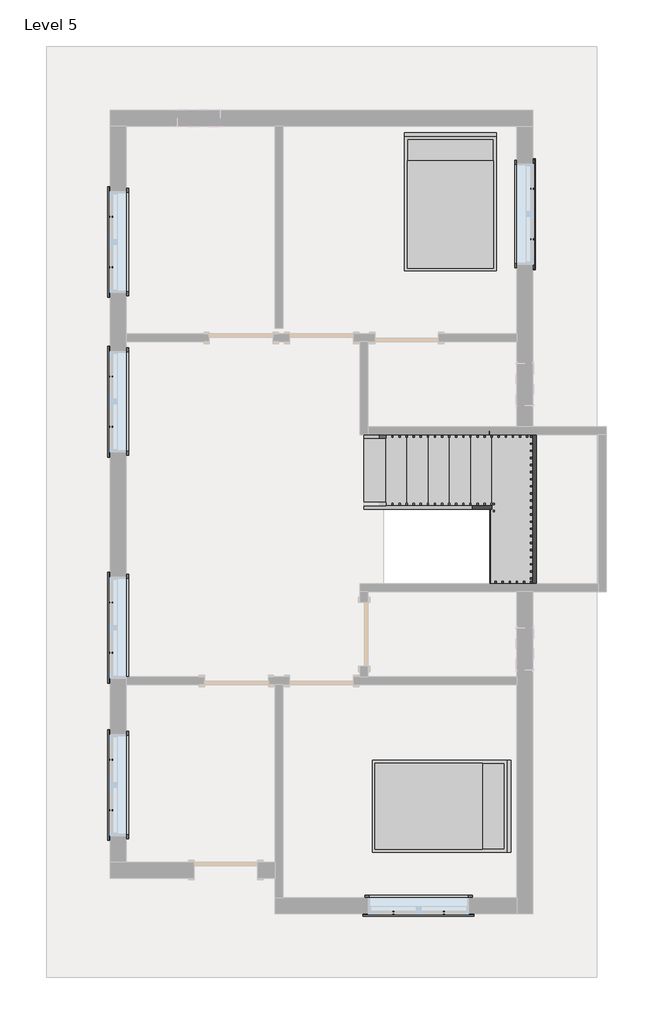
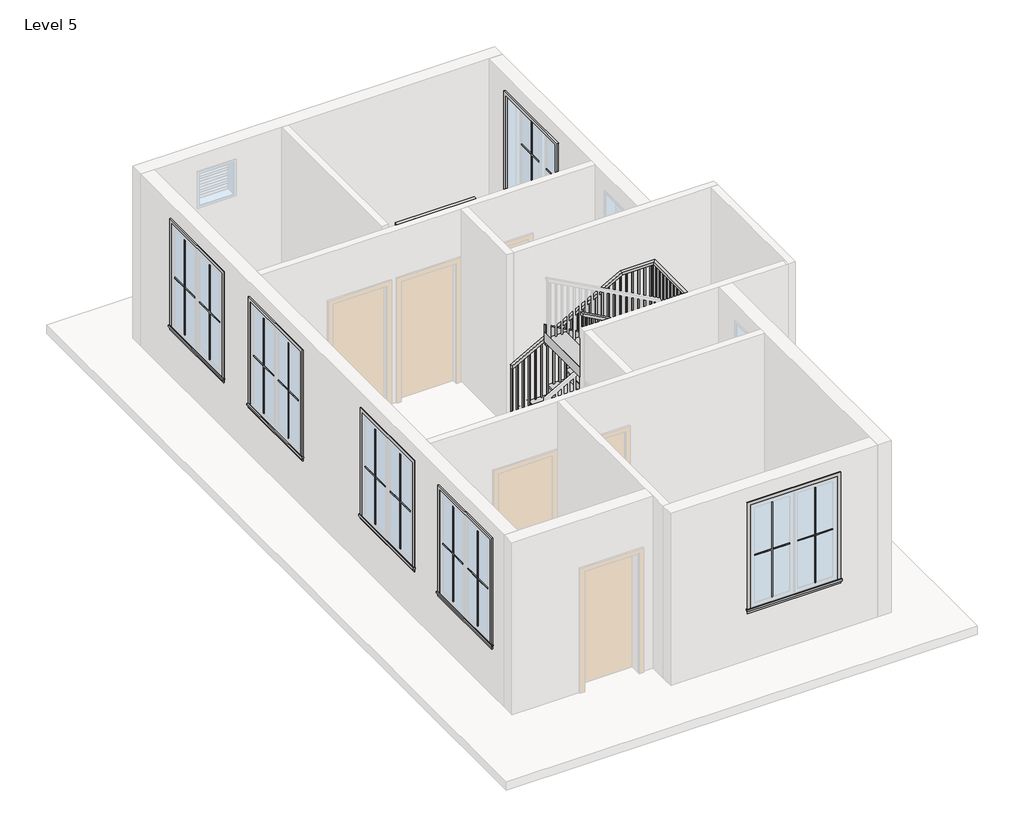
# One storey, part 2 of 2: 24 proxies, 5 members, 2 furniture elements, 1 railing, 1 stair flight.
"""IFC4 building model written with IfcOpenShell, lengths in millimetres."""

from ifc_helpers import new_model, si_unit, frame, origin, place, context, project, spatial, polyline, outline, extrude, faceted_brep, transform, mapped, element, save
from components import muntin_pattern_2x2_muntin_pattern_2x2_bff912c5, muntin_pattern_2x2_muntin_pattern_2x2_c2194282, trim_window_exterior_flat_with_sill_e04b3088, trim_window_interior_flat_picture_frame_2a7685fe, bed_17739_bed_17739_15c61121, stair_flight_cd9d6a89

model = new_model("IFC4")

# Units and contexts
model_context = context("Model", 3, world=origin())
ifc_project = project(units=[si_unit("LENGTHUNIT", "METRE", prefix="MILLI")], contexts=[model_context])

# Site, building, storey
site = spatial("IfcSite", under=ifc_project)
building = spatial("IfcBuilding", under=site)
storey = spatial("IfcBuildingStorey", under=building, Name="Level 5", Elevation=9601.2)

# Proxies
placement = place(None, origin())
muntin_pattern_2x2_muntin_pattern_2x2_shape = muntin_pattern_2x2_muntin_pattern_2x2_bff912c5(model_context)
element("IfcBuildingElementProxy", 1, Name="Muntin Pattern_2x2 : Muntin Pattern_2x2", ObjectType="Muntin Pattern_2x2 : Muntin Pattern_2x2", at=placement, inside=storey, context=model_context, shape_type="MappedRepresentation", body=[
    mapped(muntin_pattern_2x2_muntin_pattern_2x2_shape, transform((-4796.6888307, -4528.6107799, 10585.45), x_axis=(0.0, 1.0, 0.0), y_axis=(-1.0, 0.0, 0.0), z_axis=(0.0, 0.0, 1.0))),
])
element("IfcBuildingElementProxy", 2, Name="Muntin Pattern_2x2 : Muntin Pattern_2x2", ObjectType="Muntin Pattern_2x2 : Muntin Pattern_2x2", at=placement, inside=storey, context=model_context, shape_type="MappedRepresentation", body=[
    mapped(muntin_pattern_2x2_muntin_pattern_2x2_shape, transform((-4796.6888307, -2274.3607799, 10585.45), x_axis=(0.0, 1.0, 0.0), y_axis=(-1.0, 0.0, 0.0), z_axis=(0.0, 0.0, 1.0))),
])
element("IfcBuildingElementProxy", 3, Name="Muntin Pattern_2x2 : Muntin Pattern_2x2", ObjectType="Muntin Pattern_2x2 : Muntin Pattern_2x2", at=placement, inside=storey, context=model_context, shape_type="MappedRepresentation", body=[
    mapped(muntin_pattern_2x2_muntin_pattern_2x2_shape, transform((-26.2513307, -6000.2232799, 10585.45), x_axis=(-1.0, 0.0, 0.0), y_axis=(0.0, -1.0, 0.0), z_axis=(0.0, 0.0, 1.0))),
])
element("IfcBuildingElementProxy", 4, Name="Muntin Pattern_2x2 : Muntin Pattern_2x2", ObjectType="Muntin Pattern_2x2 : Muntin Pattern_2x2", at=placement, inside=storey, context=model_context, shape_type="MappedRepresentation", body=[
    mapped(muntin_pattern_2x2_muntin_pattern_2x2_shape, transform((1242.1611693, 4370.9142201, 10585.45), x_axis=(0.0, -1.0, 0.0), y_axis=(1.0, 0.0, 0.0), z_axis=(0.0, 0.0, 1.0))),
])
element("IfcBuildingElementProxy", 5, Name="Muntin Pattern_2x2 : Muntin Pattern_2x2", ObjectType="Muntin Pattern_2x2 : Muntin Pattern_2x2", at=placement, inside=storey, context=model_context, shape_type="MappedRepresentation", body=[
    mapped(muntin_pattern_2x2_muntin_pattern_2x2_shape, transform((-4796.6888307, 3250.1392201, 10585.45), x_axis=(0.0, 1.0, 0.0), y_axis=(-1.0, 0.0, 0.0), z_axis=(0.0, 0.0, 1.0))),
])
element("IfcBuildingElementProxy", 6, Name="Muntin Pattern_2x2 : Muntin Pattern_2x2", ObjectType="Muntin Pattern_2x2 : Muntin Pattern_2x2", at=placement, inside=storey, context=model_context, shape_type="MappedRepresentation", body=[
    mapped(muntin_pattern_2x2_muntin_pattern_2x2_shape, transform((-4796.6888307, 964.1392201, 10585.45), x_axis=(0.0, 1.0, 0.0), y_axis=(-1.0, 0.0, 0.0), z_axis=(0.0, 0.0, 1.0))),
])
muntin_pattern_2x2_muntin_pattern_2x2_2_shape = muntin_pattern_2x2_muntin_pattern_2x2_c2194282(model_context)
element("IfcBuildingElementProxy", 7, Name="Muntin Pattern_2x2 : Muntin Pattern_2x2", ObjectType="Muntin Pattern_2x2 : Muntin Pattern_2x2", at=placement, inside=storey, context=model_context, shape_type="MappedRepresentation", body=[
    mapped(muntin_pattern_2x2_muntin_pattern_2x2_2_shape, transform((-4796.6888307, -3807.8857799, 10585.45), x_axis=(0.0, -1.0, 0.0), y_axis=(1.0, 0.0, 0.0), z_axis=(0.0, 0.0, 1.0))),
])
element("IfcBuildingElementProxy", 8, Name="Muntin Pattern_2x2 : Muntin Pattern_2x2", ObjectType="Muntin Pattern_2x2 : Muntin Pattern_2x2", at=placement, inside=storey, context=model_context, shape_type="MappedRepresentation", body=[
    mapped(muntin_pattern_2x2_muntin_pattern_2x2_2_shape, transform((-4796.6888307, -1553.6357799, 10585.45), x_axis=(0.0, -1.0, 0.0), y_axis=(1.0, 0.0, 0.0), z_axis=(0.0, 0.0, 1.0))),
])
element("IfcBuildingElementProxy", 9, Name="Muntin Pattern_2x2 : Muntin Pattern_2x2", ObjectType="Muntin Pattern_2x2 : Muntin Pattern_2x2", at=placement, inside=storey, context=model_context, shape_type="MappedRepresentation", body=[
    mapped(muntin_pattern_2x2_muntin_pattern_2x2_2_shape, transform((-746.9763307, -6000.2232799, 10585.45), x_axis=(1.0, 0.0, 0.0), y_axis=(0.0, 1.0, 0.0), z_axis=(0.0, 0.0, 1.0))),
])
element("IfcBuildingElementProxy", 10, Name="Muntin Pattern_2x2 : Muntin Pattern_2x2", ObjectType="Muntin Pattern_2x2 : Muntin Pattern_2x2", at=placement, inside=storey, context=model_context, shape_type="MappedRepresentation", body=[
    mapped(muntin_pattern_2x2_muntin_pattern_2x2_2_shape, transform((1242.1611693, 3650.1892201, 10585.45), x_axis=(0.0, 1.0, 0.0), y_axis=(-1.0, 0.0, 0.0), z_axis=(0.0, 0.0, 1.0))),
])
element("IfcBuildingElementProxy", 11, Name="Muntin Pattern_2x2 : Muntin Pattern_2x2", ObjectType="Muntin Pattern_2x2 : Muntin Pattern_2x2", at=placement, inside=storey, context=model_context, shape_type="MappedRepresentation", body=[
    mapped(muntin_pattern_2x2_muntin_pattern_2x2_2_shape, transform((-4796.6888307, 3970.8642201, 10585.45), x_axis=(0.0, -1.0, 0.0), y_axis=(1.0, 0.0, 0.0), z_axis=(0.0, 0.0, 1.0))),
])
element("IfcBuildingElementProxy", 12, Name="Muntin Pattern_2x2 : Muntin Pattern_2x2", ObjectType="Muntin Pattern_2x2 : Muntin Pattern_2x2", at=placement, inside=storey, context=model_context, shape_type="MappedRepresentation", body=[
    mapped(muntin_pattern_2x2_muntin_pattern_2x2_2_shape, transform((-4796.6888307, 1684.8642201, 10585.45), x_axis=(0.0, -1.0, 0.0), y_axis=(1.0, 0.0, 0.0), z_axis=(0.0, 0.0, 1.0))),
])
trim_window_exterior_flat_with_sill_shape = trim_window_exterior_flat_with_sill_e04b3088(model_context)
element("IfcBuildingElementProxy", 13, Name="Trim-Window-Exterior-Flat : with Sill", ObjectType="Trim-Window-Exterior-Flat : with Sill", at=placement, inside=storey, context=model_context, shape_type="MappedRepresentation", body=[
    mapped(trim_window_exterior_flat_with_sill_shape, transform((-4806.2138307, -4168.2482799, 12344.4), x_axis=(0.0, -1.0, 0.0), y_axis=(0.0, 0.0, 1.0), z_axis=(-1.0, 0.0, 0.0))),
])
element("IfcBuildingElementProxy", 14, Name="Trim-Window-Exterior-Flat : with Sill", ObjectType="Trim-Window-Exterior-Flat : with Sill", at=placement, inside=storey, context=model_context, shape_type="MappedRepresentation", body=[
    mapped(trim_window_exterior_flat_with_sill_shape, transform((-4806.2138307, -1913.9982799, 12344.4), x_axis=(0.0, -1.0, 0.0), y_axis=(0.0, 0.0, 1.0), z_axis=(-1.0, 0.0, 0.0))),
])
element("IfcBuildingElementProxy", 15, Name="Trim-Window-Exterior-Flat : with Sill", ObjectType="Trim-Window-Exterior-Flat : with Sill", at=placement, inside=storey, context=model_context, shape_type="MappedRepresentation", body=[
    mapped(trim_window_exterior_flat_with_sill_shape, transform((-386.6138307, -6009.7482799, 12344.4), x_axis=(1.0, 0.0, 0.0), y_axis=(0.0, 0.0, 1.0), z_axis=(0.0, -1.0, 0.0))),
])
element("IfcBuildingElementProxy", 16, Name="Trim-Window-Exterior-Flat : with Sill", ObjectType="Trim-Window-Exterior-Flat : with Sill", at=placement, inside=storey, context=model_context, shape_type="MappedRepresentation", body=[
    mapped(trim_window_exterior_flat_with_sill_shape, transform((1251.6861693, 4010.5517201, 12344.4), x_axis=(0.0, 1.0, 0.0), y_axis=(0.0, 0.0, 1.0), z_axis=(1.0, 0.0, 0.0))),
])
element("IfcBuildingElementProxy", 17, Name="Trim-Window-Exterior-Flat : with Sill", ObjectType="Trim-Window-Exterior-Flat : with Sill", at=placement, inside=storey, context=model_context, shape_type="MappedRepresentation", body=[
    mapped(trim_window_exterior_flat_with_sill_shape, transform((-4806.2138307, 3610.5017201, 12344.4), x_axis=(0.0, -1.0, 0.0), y_axis=(0.0, 0.0, 1.0), z_axis=(-1.0, 0.0, 0.0))),
])
element("IfcBuildingElementProxy", 18, Name="Trim-Window-Exterior-Flat : with Sill", ObjectType="Trim-Window-Exterior-Flat : with Sill", at=placement, inside=storey, context=model_context, shape_type="MappedRepresentation", body=[
    mapped(trim_window_exterior_flat_with_sill_shape, transform((-4806.2138307, 1324.5017201, 12344.4), x_axis=(0.0, -1.0, 0.0), y_axis=(0.0, 0.0, 1.0), z_axis=(-1.0, 0.0, 0.0))),
])
trim_window_interior_flat_picture_frame_shape = trim_window_interior_flat_picture_frame_2a7685fe(model_context)
element("IfcBuildingElementProxy", 19, Name="Trim-Window-Interior-Flat : Picture Frame", ObjectType="Trim-Window-Interior-Flat : Picture Frame", at=placement, inside=storey, context=model_context, shape_type="MappedRepresentation", body=[
    mapped(trim_window_interior_flat_picture_frame_shape, transform((-4577.6138307, -4168.2482799, 12344.4), x_axis=(0.0, 1.0, 0.0), y_axis=(0.0, 0.0, 1.0), z_axis=(1.0, 0.0, 0.0))),
])
element("IfcBuildingElementProxy", 20, Name="Trim-Window-Interior-Flat : Picture Frame", ObjectType="Trim-Window-Interior-Flat : Picture Frame", at=placement, inside=storey, context=model_context, shape_type="MappedRepresentation", body=[
    mapped(trim_window_interior_flat_picture_frame_shape, transform((-4577.6138307, -1913.9982799, 12344.4), x_axis=(0.0, 1.0, 0.0), y_axis=(0.0, 0.0, 1.0), z_axis=(1.0, 0.0, 0.0))),
])
element("IfcBuildingElementProxy", 21, Name="Trim-Window-Interior-Flat : Picture Frame", ObjectType="Trim-Window-Interior-Flat : Picture Frame", at=placement, inside=storey, context=model_context, shape_type="MappedRepresentation", body=[
    mapped(trim_window_interior_flat_picture_frame_shape, transform((-386.6138307, -5781.1482799, 12344.4), x_axis=(-1.0, 0.0, 0.0), y_axis=(0.0, 0.0, 1.0), z_axis=(0.0, 1.0, 0.0))),
])
element("IfcBuildingElementProxy", 22, Name="Trim-Window-Interior-Flat : Picture Frame", ObjectType="Trim-Window-Interior-Flat : Picture Frame", at=placement, inside=storey, context=model_context, shape_type="MappedRepresentation", body=[
    mapped(trim_window_interior_flat_picture_frame_shape, transform((1023.0861693, 4010.5517201, 12344.4), x_axis=(0.0, -1.0, 0.0), y_axis=(0.0, 0.0, 1.0), z_axis=(-1.0, 0.0, 0.0))),
])
element("IfcBuildingElementProxy", 23, Name="Trim-Window-Interior-Flat : Picture Frame", ObjectType="Trim-Window-Interior-Flat : Picture Frame", at=placement, inside=storey, context=model_context, shape_type="MappedRepresentation", body=[
    mapped(trim_window_interior_flat_picture_frame_shape, transform((-4577.6138307, 3610.5017201, 12344.4), x_axis=(0.0, 1.0, 0.0), y_axis=(0.0, 0.0, 1.0), z_axis=(1.0, 0.0, 0.0))),
])
element("IfcBuildingElementProxy", 24, Name="Trim-Window-Interior-Flat : Picture Frame", ObjectType="Trim-Window-Interior-Flat : Picture Frame", at=placement, inside=storey, context=model_context, shape_type="MappedRepresentation", body=[
    mapped(trim_window_interior_flat_picture_frame_shape, transform((-4577.6138307, 1324.5017201, 12344.4), x_axis=(0.0, 1.0, 0.0), y_axis=(0.0, 0.0, 1.0), z_axis=(1.0, 0.0, 0.0))),
])

# Furniture
bed_17739_bed_17739_shape = bed_17739_bed_17739_15c61121(model_context)
element("IfcFurniture", 25, ObjectType="Bed_17739 : Bed_17739", at=placement, inside=storey, context=model_context, shape_type="MappedRepresentation", body=[
    mapped(bed_17739_bed_17739_shape, transform((70.5861693, 4162.9517201, 9601.2), x_axis=(1.0, 0.0, 0.0), y_axis=(0.0, 1.0, 0.0), z_axis=(0.0, 0.0, 1.0))),
])
element("IfcFurniture", 26, ObjectType="Bed_17739 : Bed_17739", at=placement, inside=storey, context=model_context, shape_type="MappedRepresentation", body=[
    mapped(bed_17739_bed_17739_shape, transform((-81.8138307, -4473.0482799, 9601.2), x_axis=(0.0, -1.0, 0.0), y_axis=(1.0, 0.0, 0.0), z_axis=(0.0, 0.0, 1.0))),
])

# Members
element("IfcMember", 27, ObjectType="Stringer - 2\" Width", at=placement, inside=storey, context=model_context, shape_type="SweptSolid", body=[
    extrude(outline(polyline([(9805.270617, -1167.6638307), (9601.2, -1167.6638307), (9601.2, -907.3693279), (10800.6752762, 1251.6861693), (10862.7333333, 1251.6861693), (10862.7333333, 735.7690587), (9805.270617, -1167.6638307)])), frame((0.0, 848.2517201, 0.0), z_axis=(0.0, 1.0, 0.0), x_axis=(0.0, 0.0, 1.0)), (0.0, 0.0, 1.0), 50.8),
])
element("IfcMember", 28, ObjectType="Stringer - 2\" Width", at=placement, inside=storey, context=model_context, shape_type="SweptSolid", body=[
    extrude(outline(polyline([(1251.6861693, 899.0517201), (1302.4861693, 899.0517201), (1302.4861693, -1285.3482799), (1251.6861693, -1285.3482799), (1251.6861693, 899.0517201)])), frame((0.0, 0.0, 10557.9333333), z_axis=(0.0, 0.0, 1.0), x_axis=(1.0, 0.0, 0.0)), (0.0, 0.0, 1.0), 304.8),
])
element("IfcMember", 29, ObjectType="Stringer - 2\" Width", at=placement, inside=storey, context=model_context, shape_type="SweptSolid", body=[
    extrude(outline(polyline([(10557.9333333, 1302.4861693), (10641.3539503, 1302.4861693), (12024.2428392, -1186.7138307), (11675.5641651, -1186.7138307), (10557.9333333, 825.0216665), (10557.9333333, 1302.4861693)])), frame((0.0, -1336.1482799, 0.0), z_axis=(0.0, 1.0, 0.0), x_axis=(0.0, 0.0, 1.0)), (0.0, 0.0, 1.0), 50.8),
])
element("IfcMember", 30, ObjectType="Stringer - 2\" Width", at=placement, inside=storey, context=model_context, shape_type="SweptSolid", body=[
    extrude(outline(polyline([(9805.270617, -1167.6638307), (9601.2, -1167.6638307), (9601.2, -907.3693279), (10447.8974984, 616.6861693), (10796.5761726, 616.6861693), (9805.270617, -1167.6638307)])), frame((0.0, -218.5482799, 0.0), z_axis=(0.0, 1.0, 0.0), x_axis=(0.0, 0.0, 1.0)), (0.0, 0.0, 1.0), 50.8),
])
element("IfcMember", 31, ObjectType="Stringer - 2\" Width", at=placement, inside=storey, context=model_context, shape_type="SweptSolid", body=[
    extrude(outline(polyline([(10645.453054, 667.4861693), (10994.1317281, 667.4861693), (12024.2428392, -1186.7138307), (11675.5641651, -1186.7138307), (10645.453054, 667.4861693)])), frame((0.0, -218.5482799, 0.0), z_axis=(0.0, 1.0, 0.0), x_axis=(0.0, 0.0, 1.0)), (0.0, 0.0, 1.0), 50.8),
])

# Railing
element("IfcRailing", 32, ObjectType="Handrail - Rectangular", at=placement, inside=storey, context=model_context, shape_type="SolidModel", body=[
    faceted_brep([(-1167.6638307, 848.2517201, 10684.9333333), (-1167.6638307, 848.2517201, 10626.8675836), (-1167.6638307, 797.4517201, 10626.8675836), (-1167.6638307, 797.4517201, 10684.9333333), (667.4861693, 848.2517201, 11700.9333333), (680.6099298, 848.2517201, 11650.1333333), (680.6099298, 797.4517201, 11650.1333333), (667.4861693, 797.4517201, 11700.9333333), (1251.6861693, 848.2517201, 11700.9333333), (1251.6861693, 848.2517201, 11650.1333333), (1200.8861693, 797.4517201, 11650.1333333), (1200.8861693, 797.4517201, 11700.9333333), (1251.6861693, -1285.3482799, 11700.9333333), (1251.6861693, -1285.3482799, 11650.1333333), (1200.8861693, -1234.5482799, 11650.1333333), (1200.8861693, -1234.5482799, 11700.9333333), (976.5195026, -1285.3482799, 11700.9333333), (963.5139215, -1285.3482799, 11650.1333333), (963.5139215, -1234.5482799, 11650.1333333), (976.5195026, -1234.5482799, 11700.9333333), (-1186.7138307, -1285.3482799, 12886.2666667), (-1186.7138307, -1234.5482799, 12886.2666667), (-1186.7138307, -1234.5482799, 12828.3403208), (-1186.7138307, -1285.3482799, 12828.3403208)], [[[0, 1, 2, 3]], [[1, 0, 4, 5]], [[2, 1, 5, 6]], [[3, 2, 6, 7]], [[0, 3, 7, 4]], [[5, 4, 8, 9]], [[6, 5, 9, 10]], [[7, 6, 10, 11]], [[4, 7, 11, 8]], [[9, 8, 12, 13]], [[10, 9, 13, 14]], [[11, 10, 14, 15]], [[8, 11, 15, 12]], [[13, 12, 16, 17]], [[14, 13, 17, 18]], [[15, 14, 18, 19]], [[12, 15, 19, 16]], [[20, 21, 22, 23]], [[17, 16, 20, 23]], [[18, 17, 23, 22]], [[19, 18, 22, 21]], [[16, 19, 21, 20]]]),
    extrude(outline(polyline([(12791.8060742, -1120.0388307), (11802.5333333, -1120.0388307), (11802.5333333, -1100.9888307), (12781.3677181, -1100.9888307), (12791.8060742, -1120.0388307)])), frame((0.0, -1269.4732799, 0.0), z_axis=(0.0, 1.0, 0.0), x_axis=(0.0, 0.0, 1.0)), (0.0, 0.0, 1.0), 19.05),
    extrude(outline(polyline([(12736.1348414, -1018.4388307), (11802.5333333, -1018.4388307), (11802.5333333, -999.3888307), (12725.6964852, -999.3888307), (12736.1348414, -1018.4388307)])), frame((0.0, -1269.4732799, 0.0), z_axis=(0.0, 1.0, 0.0), x_axis=(0.0, 0.0, 1.0)), (0.0, 0.0, 1.0), 19.05),
    extrude(outline(polyline([(12680.4636085, -916.8388307), (11802.5333333, -916.8388307), (11802.5333333, -897.7888307), (12670.0252523, -897.7888307), (12680.4636085, -916.8388307)])), frame((0.0, -1269.4732799, 0.0), z_axis=(0.0, 1.0, 0.0), x_axis=(0.0, 0.0, 1.0)), (0.0, 0.0, 1.0), 19.05),
    extrude(outline(polyline([(12624.7923756, -815.2388307), (11633.2, -815.2388307), (11633.2, -796.1888307), (12614.3540195, -796.1888307), (12624.7923756, -815.2388307)])), frame((0.0, -1269.4732799, 0.0), z_axis=(0.0, 1.0, 0.0), x_axis=(0.0, 0.0, 1.0)), (0.0, 0.0, 1.0), 19.05),
    extrude(outline(polyline([(12569.1211427, -713.6388307), (11633.2, -713.6388307), (11633.2, -694.5888307), (12558.6827866, -694.5888307), (12569.1211427, -713.6388307)])), frame((0.0, -1269.4732799, 0.0), z_axis=(0.0, 1.0, 0.0), x_axis=(0.0, 0.0, 1.0)), (0.0, 0.0, 1.0), 19.05),
    extrude(outline(polyline([(12513.4499099, -612.0388307), (11633.2, -612.0388307), (11633.2, -592.9888307), (12503.0115537, -592.9888307), (12513.4499099, -612.0388307)])), frame((0.0, -1269.4732799, 0.0), z_axis=(0.0, 1.0, 0.0), x_axis=(0.0, 0.0, 1.0)), (0.0, 0.0, 1.0), 19.05),
    extrude(outline(polyline([(12457.778677, -510.4388307), (11463.8666667, -510.4388307), (11463.8666667, -491.3888307), (12447.3403208, -491.3888307), (12457.778677, -510.4388307)])), frame((0.0, -1269.4732799, 0.0), z_axis=(0.0, 1.0, 0.0), x_axis=(0.0, 0.0, 1.0)), (0.0, 0.0, 1.0), 19.05),
    extrude(outline(polyline([(12402.1074441, -408.8388307), (11463.8666667, -408.8388307), (11463.8666667, -389.7888307), (12391.6690879, -389.7888307), (12402.1074441, -408.8388307)])), frame((0.0, -1269.4732799, 0.0), z_axis=(0.0, 1.0, 0.0), x_axis=(0.0, 0.0, 1.0)), (0.0, 0.0, 1.0), 19.05),
    extrude(outline(polyline([(12346.4362112, -307.2388307), (11463.8666667, -307.2388307), (11463.8666667, -288.1888307), (12335.9978551, -288.1888307), (12346.4362112, -307.2388307)])), frame((0.0, -1269.4732799, 0.0), z_axis=(0.0, 1.0, 0.0), x_axis=(0.0, 0.0, 1.0)), (0.0, 0.0, 1.0), 19.05),
    extrude(outline(polyline([(12290.7649784, -205.6388307), (11294.5333333, -205.6388307), (11294.5333333, -186.5888307), (12280.3266222, -186.5888307), (12290.7649784, -205.6388307)])), frame((0.0, -1269.4732799, 0.0), z_axis=(0.0, 1.0, 0.0), x_axis=(0.0, 0.0, 1.0)), (0.0, 0.0, 1.0), 19.05),
    extrude(outline(polyline([(12235.0937455, -104.0388307), (11294.5333333, -104.0388307), (11294.5333333, -84.9888307), (12224.6553893, -84.9888307), (12235.0937455, -104.0388307)])), frame((0.0, -1269.4732799, 0.0), z_axis=(0.0, 1.0, 0.0), x_axis=(0.0, 0.0, 1.0)), (0.0, 0.0, 1.0), 19.05),
    extrude(outline(polyline([(12179.4225126, -2.4388307), (11294.5333333, -2.4388307), (11294.5333333, 16.6111693), (12168.9841564, 16.6111693), (12179.4225126, -2.4388307)])), frame((0.0, -1269.4732799, 0.0), z_axis=(0.0, 1.0, 0.0), x_axis=(0.0, 0.0, 1.0)), (0.0, 0.0, 1.0), 19.05),
    extrude(outline(polyline([(12123.7512797, 99.1611693), (11125.2, 99.1611693), (11125.2, 118.2111693), (12113.3129236, 118.2111693), (12123.7512797, 99.1611693)])), frame((0.0, -1269.4732799, 0.0), z_axis=(0.0, 1.0, 0.0), x_axis=(0.0, 0.0, 1.0)), (0.0, 0.0, 1.0), 19.05),
    extrude(outline(polyline([(12068.0800469, 200.7611693), (11125.2, 200.7611693), (11125.2, 219.8111693), (12057.6416907, 219.8111693), (12068.0800469, 200.7611693)])), frame((0.0, -1269.4732799, 0.0), z_axis=(0.0, 1.0, 0.0), x_axis=(0.0, 0.0, 1.0)), (0.0, 0.0, 1.0), 19.05),
    extrude(outline(polyline([(12012.408814, 302.3611693), (11125.2, 302.3611693), (11125.2, 321.4111693), (12001.9704578, 321.4111693), (12012.408814, 302.3611693)])), frame((0.0, -1269.4732799, 0.0), z_axis=(0.0, 1.0, 0.0), x_axis=(0.0, 0.0, 1.0)), (0.0, 0.0, 1.0), 19.05),
    extrude(outline(polyline([(11956.7375811, 403.9611693), (10955.8666667, 403.9611693), (10955.8666667, 423.0111693), (11946.2992249, 423.0111693), (11956.7375811, 403.9611693)])), frame((0.0, -1269.4732799, 0.0), z_axis=(0.0, 1.0, 0.0), x_axis=(0.0, 0.0, 1.0)), (0.0, 0.0, 1.0), 19.05),
    extrude(outline(polyline([(11901.0663482, 505.5611693), (10955.8666667, 505.5611693), (10955.8666667, 524.6111693), (11890.6279921, 524.6111693), (11901.0663482, 505.5611693)])), frame((0.0, -1269.4732799, 0.0), z_axis=(0.0, 1.0, 0.0), x_axis=(0.0, 0.0, 1.0)), (0.0, 0.0, 1.0), 19.05),
    extrude(outline(polyline([(11845.3951153, 607.1611693), (10955.8666667, 607.1611693), (10955.8666667, 626.2111693), (11834.9567592, 626.2111693), (11845.3951153, 607.1611693)])), frame((0.0, -1269.4732799, 0.0), z_axis=(0.0, 1.0, 0.0), x_axis=(0.0, 0.0, 1.0)), (0.0, 0.0, 1.0), 19.05),
    extrude(outline(polyline([(11789.7238825, 708.7611693), (10786.5333333, 708.7611693), (10786.5333333, 727.8111693), (11779.2855263, 727.8111693), (11789.7238825, 708.7611693)])), frame((0.0, -1269.4732799, 0.0), z_axis=(0.0, 1.0, 0.0), x_axis=(0.0, 0.0, 1.0)), (0.0, 0.0, 1.0), 19.05),
    extrude(outline(polyline([(11734.0526496, 810.3611693), (10786.5333333, 810.3611693), (10786.5333333, 829.4111693), (11723.6142934, 829.4111693), (11734.0526496, 810.3611693)])), frame((0.0, -1269.4732799, 0.0), z_axis=(0.0, 1.0, 0.0), x_axis=(0.0, 0.0, 1.0)), (0.0, 0.0, 1.0), 19.05),
    extrude(outline(polyline([(11678.3814167, 911.9611693), (10786.5333333, 911.9611693), (10786.5333333, 931.0111693), (11667.9430606, 931.0111693), (11678.3814167, 911.9611693)])), frame((0.0, -1269.4732799, 0.0), z_axis=(0.0, 1.0, 0.0), x_axis=(0.0, 0.0, 1.0)), (0.0, 0.0, 1.0), 19.05),
    extrude(outline(polyline([(1032.6111693, -1269.4732799), (1013.5611693, -1269.4732799), (1013.5611693, -1250.4232799), (1032.6111693, -1250.4232799), (1032.6111693, -1269.4732799)])), frame((0.0, 0.0, 10786.5333333), z_axis=(0.0, 0.0, 1.0), x_axis=(1.0, 0.0, 0.0)), (0.0, 0.0, 1.0), 863.6),
    extrude(outline(polyline([(1134.2111693, -1269.4732799), (1115.1611693, -1269.4732799), (1115.1611693, -1250.4232799), (1134.2111693, -1250.4232799), (1134.2111693, -1269.4732799)])), frame((0.0, 0.0, 10786.5333333), z_axis=(0.0, 0.0, 1.0), x_axis=(1.0, 0.0, 0.0)), (0.0, 0.0, 1.0), 863.6),
    extrude(outline(polyline([(1235.8111693, -1199.6232799), (1235.8111693, -1218.6732799), (1216.7611693, -1218.6732799), (1216.7611693, -1199.6232799), (1235.8111693, -1199.6232799)])), frame((0.0, 0.0, 10786.5333333), z_axis=(0.0, 0.0, 1.0), x_axis=(1.0, 0.0, 0.0)), (0.0, 0.0, 1.0), 863.6),
    extrude(outline(polyline([(1235.8111693, -1098.0232799), (1235.8111693, -1117.0732799), (1216.7611693, -1117.0732799), (1216.7611693, -1098.0232799), (1235.8111693, -1098.0232799)])), frame((0.0, 0.0, 10786.5333333), z_axis=(0.0, 0.0, 1.0), x_axis=(1.0, 0.0, 0.0)), (0.0, 0.0, 1.0), 863.6),
    extrude(outline(polyline([(1235.8111693, -996.4232799), (1235.8111693, -1015.4732799), (1216.7611693, -1015.4732799), (1216.7611693, -996.4232799), (1235.8111693, -996.4232799)])), frame((0.0, 0.0, 10786.5333333), z_axis=(0.0, 0.0, 1.0), x_axis=(1.0, 0.0, 0.0)), (0.0, 0.0, 1.0), 863.6),
    extrude(outline(polyline([(1235.8111693, -894.8232799), (1235.8111693, -913.8732799), (1216.7611693, -913.8732799), (1216.7611693, -894.8232799), (1235.8111693, -894.8232799)])), frame((0.0, 0.0, 10786.5333333), z_axis=(0.0, 0.0, 1.0), x_axis=(1.0, 0.0, 0.0)), (0.0, 0.0, 1.0), 863.6),
    extrude(outline(polyline([(1235.8111693, -793.2232799), (1235.8111693, -812.2732799), (1216.7611693, -812.2732799), (1216.7611693, -793.2232799), (1235.8111693, -793.2232799)])), frame((0.0, 0.0, 10786.5333333), z_axis=(0.0, 0.0, 1.0), x_axis=(1.0, 0.0, 0.0)), (0.0, 0.0, 1.0), 863.6),
    extrude(outline(polyline([(1235.8111693, -691.6232799), (1235.8111693, -710.6732799), (1216.7611693, -710.6732799), (1216.7611693, -691.6232799), (1235.8111693, -691.6232799)])), frame((0.0, 0.0, 10786.5333333), z_axis=(0.0, 0.0, 1.0), x_axis=(1.0, 0.0, 0.0)), (0.0, 0.0, 1.0), 863.6),
    extrude(outline(polyline([(1235.8111693, -590.0232799), (1235.8111693, -609.0732799), (1216.7611693, -609.0732799), (1216.7611693, -590.0232799), (1235.8111693, -590.0232799)])), frame((0.0, 0.0, 10786.5333333), z_axis=(0.0, 0.0, 1.0), x_axis=(1.0, 0.0, 0.0)), (0.0, 0.0, 1.0), 863.6),
    extrude(outline(polyline([(1235.8111693, -488.4232799), (1235.8111693, -507.4732799), (1216.7611693, -507.4732799), (1216.7611693, -488.4232799), (1235.8111693, -488.4232799)])), frame((0.0, 0.0, 10786.5333333), z_axis=(0.0, 0.0, 1.0), x_axis=(1.0, 0.0, 0.0)), (0.0, 0.0, 1.0), 863.6),
    extrude(outline(polyline([(1235.8111693, -386.8232799), (1235.8111693, -405.8732799), (1216.7611693, -405.8732799), (1216.7611693, -386.8232799), (1235.8111693, -386.8232799)])), frame((0.0, 0.0, 10786.5333333), z_axis=(0.0, 0.0, 1.0), x_axis=(1.0, 0.0, 0.0)), (0.0, 0.0, 1.0), 863.6),
    extrude(outline(polyline([(1235.8111693, -285.2232799), (1235.8111693, -304.2732799), (1216.7611693, -304.2732799), (1216.7611693, -285.2232799), (1235.8111693, -285.2232799)])), frame((0.0, 0.0, 10786.5333333), z_axis=(0.0, 0.0, 1.0), x_axis=(1.0, 0.0, 0.0)), (0.0, 0.0, 1.0), 863.6),
    extrude(outline(polyline([(1235.8111693, -183.6232799), (1235.8111693, -202.6732799), (1216.7611693, -202.6732799), (1216.7611693, -183.6232799), (1235.8111693, -183.6232799)])), frame((0.0, 0.0, 10786.5333333), z_axis=(0.0, 0.0, 1.0), x_axis=(1.0, 0.0, 0.0)), (0.0, 0.0, 1.0), 863.6),
    extrude(outline(polyline([(1235.8111693, -82.0232799), (1235.8111693, -101.0732799), (1216.7611693, -101.0732799), (1216.7611693, -82.0232799), (1235.8111693, -82.0232799)])), frame((0.0, 0.0, 10786.5333333), z_axis=(0.0, 0.0, 1.0), x_axis=(1.0, 0.0, 0.0)), (0.0, 0.0, 1.0), 863.6),
    extrude(outline(polyline([(1235.8111693, 19.5767201), (1235.8111693, 0.5267201), (1216.7611693, 0.5267201), (1216.7611693, 19.5767201), (1235.8111693, 19.5767201)])), frame((0.0, 0.0, 10786.5333333), z_axis=(0.0, 0.0, 1.0), x_axis=(1.0, 0.0, 0.0)), (0.0, 0.0, 1.0), 863.6),
    extrude(outline(polyline([(1235.8111693, 121.1767201), (1235.8111693, 102.1267201), (1216.7611693, 102.1267201), (1216.7611693, 121.1767201), (1235.8111693, 121.1767201)])), frame((0.0, 0.0, 10786.5333333), z_axis=(0.0, 0.0, 1.0), x_axis=(1.0, 0.0, 0.0)), (0.0, 0.0, 1.0), 863.6),
    extrude(outline(polyline([(1235.8111693, 222.7767201), (1235.8111693, 203.7267201), (1216.7611693, 203.7267201), (1216.7611693, 222.7767201), (1235.8111693, 222.7767201)])), frame((0.0, 0.0, 10786.5333333), z_axis=(0.0, 0.0, 1.0), x_axis=(1.0, 0.0, 0.0)), (0.0, 0.0, 1.0), 863.6),
    extrude(outline(polyline([(1235.8111693, 324.3767201), (1235.8111693, 305.3267201), (1216.7611693, 305.3267201), (1216.7611693, 324.3767201), (1235.8111693, 324.3767201)])), frame((0.0, 0.0, 10786.5333333), z_axis=(0.0, 0.0, 1.0), x_axis=(1.0, 0.0, 0.0)), (0.0, 0.0, 1.0), 863.6),
    extrude(outline(polyline([(1235.8111693, 425.9767201), (1235.8111693, 406.9267201), (1216.7611693, 406.9267201), (1216.7611693, 425.9767201), (1235.8111693, 425.9767201)])), frame((0.0, 0.0, 10786.5333333), z_axis=(0.0, 0.0, 1.0), x_axis=(1.0, 0.0, 0.0)), (0.0, 0.0, 1.0), 863.6),
    extrude(outline(polyline([(1235.8111693, 527.5767201), (1235.8111693, 508.5267201), (1216.7611693, 508.5267201), (1216.7611693, 527.5767201), (1235.8111693, 527.5767201)])), frame((0.0, 0.0, 10786.5333333), z_axis=(0.0, 0.0, 1.0), x_axis=(1.0, 0.0, 0.0)), (0.0, 0.0, 1.0), 863.6),
    extrude(outline(polyline([(1235.8111693, 629.1767201), (1235.8111693, 610.1267201), (1216.7611693, 610.1267201), (1216.7611693, 629.1767201), (1235.8111693, 629.1767201)])), frame((0.0, 0.0, 10786.5333333), z_axis=(0.0, 0.0, 1.0), x_axis=(1.0, 0.0, 0.0)), (0.0, 0.0, 1.0), 863.6),
    extrude(outline(polyline([(1235.8111693, 730.7767201), (1235.8111693, 711.7267201), (1216.7611693, 711.7267201), (1216.7611693, 730.7767201), (1235.8111693, 730.7767201)])), frame((0.0, 0.0, 10786.5333333), z_axis=(0.0, 0.0, 1.0), x_axis=(1.0, 0.0, 0.0)), (0.0, 0.0, 1.0), 863.6),
    extrude(outline(polyline([(1159.6111693, 832.3767201), (1178.6611693, 832.3767201), (1178.6611693, 813.3267201), (1159.6111693, 813.3267201), (1159.6111693, 832.3767201)])), frame((0.0, 0.0, 10786.5333333), z_axis=(0.0, 0.0, 1.0), x_axis=(1.0, 0.0, 0.0)), (0.0, 0.0, 1.0), 863.6),
    extrude(outline(polyline([(1058.0111693, 832.3767201), (1077.0611693, 832.3767201), (1077.0611693, 813.3267201), (1058.0111693, 813.3267201), (1058.0111693, 832.3767201)])), frame((0.0, 0.0, 10786.5333333), z_axis=(0.0, 0.0, 1.0), x_axis=(1.0, 0.0, 0.0)), (0.0, 0.0, 1.0), 863.6),
    extrude(outline(polyline([(956.4111693, 832.3767201), (975.4611693, 832.3767201), (975.4611693, 813.3267201), (956.4111693, 813.3267201), (956.4111693, 832.3767201)])), frame((0.0, 0.0, 10786.5333333), z_axis=(0.0, 0.0, 1.0), x_axis=(1.0, 0.0, 0.0)), (0.0, 0.0, 1.0), 863.6),
    extrude(outline(polyline([(854.8111693, 832.3767201), (873.8611693, 832.3767201), (873.8611693, 813.3267201), (854.8111693, 813.3267201), (854.8111693, 832.3767201)])), frame((0.0, 0.0, 10786.5333333), z_axis=(0.0, 0.0, 1.0), x_axis=(1.0, 0.0, 0.0)), (0.0, 0.0, 1.0), 863.6),
    extrude(outline(polyline([(753.2111693, 832.3767201), (772.2611693, 832.3767201), (772.2611693, 813.3267201), (753.2111693, 813.3267201), (753.2111693, 832.3767201)])), frame((0.0, 0.0, 10786.5333333), z_axis=(0.0, 0.0, 1.0), x_axis=(1.0, 0.0, 0.0)), (0.0, 0.0, 1.0), 863.6),
    extrude(outline(polyline([(11634.0786562, 651.6111693), (10617.2, 651.6111693), (10617.2, 670.6611693), (11644.625369, 670.6611693), (11634.0786562, 651.6111693)])), frame((0.0, 813.3267201, 0.0), z_axis=(0.0, 1.0, 0.0), x_axis=(0.0, 0.0, 1.0)), (0.0, 0.0, 1.0), 19.05),
    extrude(outline(polyline([(11577.8295213, 550.0111693), (10617.2, 550.0111693), (10617.2, 569.0611693), (11588.3762341, 569.0611693), (11577.8295213, 550.0111693)])), frame((0.0, 813.3267201, 0.0), z_axis=(0.0, 1.0, 0.0), x_axis=(0.0, 0.0, 1.0)), (0.0, 0.0, 1.0), 19.05),
    extrude(outline(polyline([(11521.5803863, 448.4111693), (10617.2, 448.4111693), (10617.2, 467.4611693), (11532.1270991, 467.4611693), (11521.5803863, 448.4111693)])), frame((0.0, 813.3267201, 0.0), z_axis=(0.0, 1.0, 0.0), x_axis=(0.0, 0.0, 1.0)), (0.0, 0.0, 1.0), 19.05),
    extrude(outline(polyline([(11465.3312514, 346.8111693), (10447.8666667, 346.8111693), (10447.8666667, 365.8611693), (11475.8779642, 365.8611693), (11465.3312514, 346.8111693)])), frame((0.0, 813.3267201, 0.0), z_axis=(0.0, 1.0, 0.0), x_axis=(0.0, 0.0, 1.0)), (0.0, 0.0, 1.0), 19.05),
    extrude(outline(polyline([(11409.0821164, 245.2111693), (10447.8666667, 245.2111693), (10447.8666667, 264.2611693), (11419.6288292, 264.2611693), (11409.0821164, 245.2111693)])), frame((0.0, 813.3267201, 0.0), z_axis=(0.0, 1.0, 0.0), x_axis=(0.0, 0.0, 1.0)), (0.0, 0.0, 1.0), 19.05),
    extrude(outline(polyline([(11352.8329815, 143.6111693), (10447.8666667, 143.6111693), (10447.8666667, 162.6611693), (11363.3796943, 162.6611693), (11352.8329815, 143.6111693)])), frame((0.0, 813.3267201, 0.0), z_axis=(0.0, 1.0, 0.0), x_axis=(0.0, 0.0, 1.0)), (0.0, 0.0, 1.0), 19.05),
    extrude(outline(polyline([(11296.5838465, 42.0111693), (10278.5333333, 42.0111693), (10278.5333333, 61.0611693), (11307.1305593, 61.0611693), (11296.5838465, 42.0111693)])), frame((0.0, 813.3267201, 0.0), z_axis=(0.0, 1.0, 0.0), x_axis=(0.0, 0.0, 1.0)), (0.0, 0.0, 1.0), 19.05),
    extrude(outline(polyline([(11240.3347116, -59.5888307), (10278.5333333, -59.5888307), (10278.5333333, -40.5388307), (11250.8814244, -40.5388307), (11240.3347116, -59.5888307)])), frame((0.0, 813.3267201, 0.0), z_axis=(0.0, 1.0, 0.0), x_axis=(0.0, 0.0, 1.0)), (0.0, 0.0, 1.0), 19.05),
    extrude(outline(polyline([(11184.0855766, -161.1888307), (10278.5333333, -161.1888307), (10278.5333333, -142.1388307), (11194.6322895, -142.1388307), (11184.0855766, -161.1888307)])), frame((0.0, 813.3267201, 0.0), z_axis=(0.0, 1.0, 0.0), x_axis=(0.0, 0.0, 1.0)), (0.0, 0.0, 1.0), 19.05),
    extrude(outline(polyline([(11127.8364417, -262.7888307), (10109.2, -262.7888307), (10109.2, -243.7388307), (11138.3831545, -243.7388307), (11127.8364417, -262.7888307)])), frame((0.0, 813.3267201, 0.0), z_axis=(0.0, 1.0, 0.0), x_axis=(0.0, 0.0, 1.0)), (0.0, 0.0, 1.0), 19.05),
    extrude(outline(polyline([(11071.5873068, -364.3888307), (10109.2, -364.3888307), (10109.2, -345.3388307), (11082.1340196, -345.3388307), (11071.5873068, -364.3888307)])), frame((0.0, 813.3267201, 0.0), z_axis=(0.0, 1.0, 0.0), x_axis=(0.0, 0.0, 1.0)), (0.0, 0.0, 1.0), 19.05),
    extrude(outline(polyline([(11015.3381718, -465.9888307), (10109.2, -465.9888307), (10109.2, -446.9388307), (11025.8848846, -446.9388307), (11015.3381718, -465.9888307)])), frame((0.0, 813.3267201, 0.0), z_axis=(0.0, 1.0, 0.0), x_axis=(0.0, 0.0, 1.0)), (0.0, 0.0, 1.0), 19.05),
    extrude(outline(polyline([(10959.0890369, -567.5888307), (9939.8666667, -567.5888307), (9939.8666667, -548.5388307), (10969.6357497, -548.5388307), (10959.0890369, -567.5888307)])), frame((0.0, 813.3267201, 0.0), z_axis=(0.0, 1.0, 0.0), x_axis=(0.0, 0.0, 1.0)), (0.0, 0.0, 1.0), 19.05),
    extrude(outline(polyline([(10902.8399019, -669.1888307), (9939.8666667, -669.1888307), (9939.8666667, -650.1388307), (10913.3866147, -650.1388307), (10902.8399019, -669.1888307)])), frame((0.0, 813.3267201, 0.0), z_axis=(0.0, 1.0, 0.0), x_axis=(0.0, 0.0, 1.0)), (0.0, 0.0, 1.0), 19.05),
    extrude(outline(polyline([(10846.590767, -770.7888307), (9939.8666667, -770.7888307), (9939.8666667, -751.7388307), (10857.1374798, -751.7388307), (10846.590767, -770.7888307)])), frame((0.0, 813.3267201, 0.0), z_axis=(0.0, 1.0, 0.0), x_axis=(0.0, 0.0, 1.0)), (0.0, 0.0, 1.0), 19.05),
    extrude(outline(polyline([(10790.341632, -872.3888307), (9770.5333333, -872.3888307), (9770.5333333, -853.3388307), (10800.8883448, -853.3388307), (10790.341632, -872.3888307)])), frame((0.0, 813.3267201, 0.0), z_axis=(0.0, 1.0, 0.0), x_axis=(0.0, 0.0, 1.0)), (0.0, 0.0, 1.0), 19.05),
    extrude(outline(polyline([(10734.0924971, -973.9888307), (9770.5333333, -973.9888307), (9770.5333333, -954.9388307), (10744.6392099, -954.9388307), (10734.0924971, -973.9888307)])), frame((0.0, 813.3267201, 0.0), z_axis=(0.0, 1.0, 0.0), x_axis=(0.0, 0.0, 1.0)), (0.0, 0.0, 1.0), 19.05),
    extrude(outline(polyline([(10677.8433621, -1075.5888307), (9770.5333333, -1075.5888307), (9770.5333333, -1056.5388307), (10688.3900749, -1056.5388307), (10677.8433621, -1075.5888307)])), frame((0.0, 813.3267201, 0.0), z_axis=(0.0, 1.0, 0.0), x_axis=(0.0, 0.0, 1.0)), (0.0, 0.0, 1.0), 19.05),
    extrude(outline(polyline([(1235.8111693, -1250.4232799), (1235.8111693, -1269.4732799), (1216.7611693, -1269.4732799), (1216.7611693, -1250.4232799), (1235.8111693, -1250.4232799)])), frame((0.0, 0.0, 10786.5333333), z_axis=(0.0, 0.0, 1.0), x_axis=(1.0, 0.0, 0.0)), (0.0, 0.0, 1.0), 863.6),
    extrude(outline(polyline([(1216.7611693, 832.3767201), (1235.8111693, 832.3767201), (1235.8111693, 813.3267201), (1216.7611693, 813.3267201), (1216.7611693, 832.3767201)])), frame((0.0, 0.0, 10786.5333333), z_axis=(0.0, 0.0, 1.0), x_axis=(1.0, 0.0, 0.0)), (0.0, 0.0, 1.0), 863.6),
    extrude(outline(polyline([(12828.3403208, -1186.7138307), (11802.5333333, -1186.7138307), (11802.5333333, -1167.6638307), (12817.9019647, -1167.6638307), (12828.3403208, -1186.7138307)])), frame((0.0, -1269.4732799, 0.0), z_axis=(0.0, 1.0, 0.0), x_axis=(0.0, 0.0, 1.0)), (0.0, 0.0, 1.0), 19.05),
    extrude(outline(polyline([(10626.8675836, -1167.6638307), (9770.5333333, -1167.6638307), (9770.5333333, -1148.6138307), (10637.4142964, -1148.6138307), (10626.8675836, -1167.6638307)])), frame((0.0, 813.3267201, 0.0), z_axis=(0.0, 1.0, 0.0), x_axis=(0.0, 0.0, 1.0)), (0.0, 0.0, 1.0), 19.05),
])

# Stair flight
stair_flight_shape = stair_flight_cd9d6a89(model_context)
element("IfcStairFlight", 33, ObjectType="2\" Tread 1\" Nosing 1/4\" Riser", at=placement, inside=storey, context=model_context, shape_type="MappedRepresentation", body=[
    mapped(stair_flight_shape, transform((0.0, 0.0, 0.0), x_axis=(1.0, 0.0, 0.0), y_axis=(0.0, 1.0, 0.0), z_axis=(0.0, 0.0, 1.0))),
])

save(model, "model.ifc")

# Revit data of these elements
# Type "Muntin Pattern_2x2 : Muntin Pattern_2x2"
#   Width [instance default] = 4' - 0"
#   Thickness = 0' - 0 1/2"
#   Height [instance default] = 4' - 0"
#   Distance = 0' - 0 3/4"
#   Interior Material [instance default] = none
#   Exterior Material [instance default] = none
#   Default Elevation = 0
# Type "Trim-Window-Exterior-Flat : with Sill"
#   Trim Width = 0' - 2 1/4"
#   Trim Thickness_Picture Frame = 0' - 1 1/4"
#   Trim Thickness_with Sill = 0' - 0 3/4"
#   Sill Thickness = 0' - 1 1/4"
#   Opening Width [instance default] = 2' - 0"
#   Opening Height [instance default] = 3' - 0"
#   Default Elevation = 4' - 0"
#   Sill = yes
#   Picture Frame = no
#   Trim Material [instance default] = none
# Type "Trim-Window-Interior-Flat : Picture Frame"
#   Trim Thickness_Picture Frame = 0' - 1 1/4"
#   Trim Width = 0' - 2 1/4"
#   Trim Thickness_with Sill = 0' - 0 3/4"
#   Sill Thickness = 0' - 1 1/4"
#   Opening Width [instance default] = 2' - 0"
#   Opening Height [instance default] = 3' - 0"
#   Default Elevation = 4' - 0"
#   Sill = no
#   Picture Frame = yes
#   Trim Material [instance default] = none
# Type "Bed_17739 : Bed_17739"
#   Default Elevation = 0
# Type "Handrail - Rectangular"
#   Assembly Code = "C2010400"
#   built-in parameter 1008612 = 0.0416667 (stored number, unit not read)
#   built-in parameter 1008611 = 0.0416667 (stored number, unit not read)
#   built-in parameter 1008609 = 0.333333 (stored number, unit not read)
#   built-in parameter 1008604 = 0.166667 (stored number, unit not read)
#   built-in parameter 1008603 = 0.166667 (stored number, unit not read)
#   Railing Height = 3' - 0"
#   built-in parameter 1008630 = 2
#   built-in parameter 1008610 = 2
#   built-in parameter 1008618 = Baluster - Square : 3/4"
# Elements 1, 2, 3, 4, 5, 6, 7, 8, 9, 10, 11, 12 (IfcBuildingElementProxy, "Muntin Pattern_2x2 : Muntin Pattern_2x2")
#   Width = 1' - 11 1/8"
#   Height = 5' - 6 1/2"
#   Interior Material = Wood - Stained
#   Exterior Material = Clad - White
#   Phase Created = New Construction
#   Materials on its faces: "Clad - White", "Wood - Stained"
# Elements 13, 14, 15, 16, 17, 18 (IfcBuildingElementProxy, "Trim-Window-Exterior-Flat : with Sill")
#   Opening Width = 4' - 9"
#   Opening Height = 6' - 0"
#   Trim Material = Clad - White
#   Phase Created = New Construction
#   Materials on its faces: "Clad - White"
# Elements 19, 20, 21, 22, 23, 24 (IfcBuildingElementProxy, "Trim-Window-Interior-Flat : Picture Frame")
#   Opening Width = 4' - 9"
#   Opening Height = 6' - 0"
#   Trim Material = Wood - Stained
#   Phase Created = New Construction
#   Materials on its faces: "Wood - Stained"
# Elements 25, 26 (IfcFurniture, "Bed_17739 : Bed_17739")
#   Phase Created = New Construction
#   Materials on its faces: "legs", "sheets", "bed frame", "Blanket"
# Elements 27, 28, 29, 30, 31 (IfcMember, "Stringer - 2\" Width")
#   Phase Created = New Construction
# Element 32 (IfcRailing, "Handrail - Rectangular")
#   Phase Created = New Construction
# Element 33 (IfcStairFlight, "2\" Tread 1\" Nosing 1/4\" Riser")
#   Phase Created = New Construction
# Materials
#   "Clad - White": class "Wood", colour RGB 242 242 238, transparency 0, Cost = 0
#   "Wood - Stained": class "Wood", colour RGB 224 178 126, transparency 0, Cost = 0
#   "legs": colour RGB 90 73 37, transparency 0, Cost = 0
#   "sheets": colour RGB 200 195 176, transparency 0, Cost = 0
#   "bed frame": colour RGB 90 73 37, transparency 0, Cost = 0
#   "Blanket": class "System", colour RGB 59 0 1, transparency 0, Cost = 0
